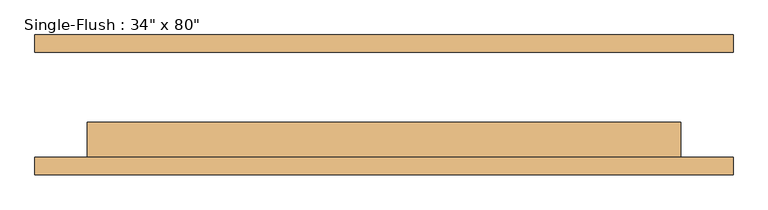
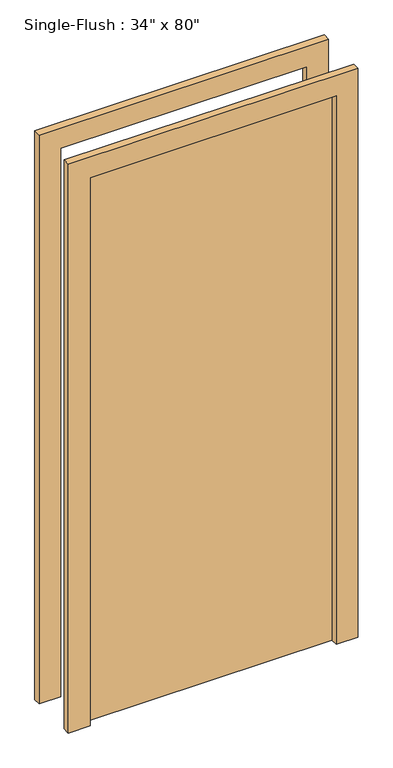
"""IFC4 building model written with IfcOpenShell, lengths in millimetres: door geometry."""

from ifc_helpers import new_model, si_unit, frame, origin, origin_with_axes, place, context, project, spatial, polyline, outline, extrude, source, transform, mapped, element, save


def door_706f0888(model_context):
    return source(origin(), model_context, "Body", "SweptSolid", [
        extrude(outline(polyline([(2108.2, -508.0), (0.0, -508.0), (0.0, -431.8), (2032.0, -431.8), (2032.0, 431.8), (0.0, 431.8), (0.0, 508.0), (2108.2, 508.0), (2108.2, -508.0)])), frame((0.0, -101.6, 0.0), z_axis=(0.0, 1.0, 0.0), x_axis=(0.0, 0.0, 1.0)), (0.0, 0.0, 1.0), 25.4),
        extrude(outline(polyline([(2108.2, 508.0), (2108.2, -508.0), (0.0, -508.0), (0.0, -431.8), (2032.0, -431.8), (2032.0, 431.8), (0.0, 431.8), (0.0, 508.0), (2108.2, 508.0)])), frame((0.0, 76.2, 0.0), z_axis=(0.0, 1.0, 0.0), x_axis=(0.0, 0.0, 1.0)), (0.0, 0.0, 1.0), 25.4),
        extrude(outline(polyline([(431.8, -25.4), (431.8, -76.2), (-431.8, -76.2), (-431.8, -25.4), (431.8, -25.4)])), origin_with_axes(), (0.0, 0.0, 1.0), 2032.0),
    ])


if __name__ == "__main__":
    model = new_model("IFC4")
    model_context = context("Model", 3, world=origin())
    ifc_project = project(units=[si_unit("LENGTHUNIT", "METRE", prefix="MILLI")], contexts=[model_context])
    site = spatial("IfcSite", under=ifc_project)
    building = spatial("IfcBuilding", under=site)
    placement = place(None, origin())
    door_shape = door_706f0888(model_context)
    element("IfcDoor", 1, ObjectType="Single-Flush : 34\" x 80\"", at=placement, inside=building, context=model_context, shape_type="MappedRepresentation", body=[
        mapped(door_shape, transform((0.0, 0.0, 0.0), x_axis=(1.0, 0.0, 0.0), y_axis=(0.0, 1.0, 0.0), z_axis=(0.0, 0.0, 1.0))),
    ])
    save(model, "model.ifc")

# Revit data of these elements
# Type "Single-Flush : 34\" x 80\""
#   Type Mark = "7"
#   Construction Type Id = "MDOOR"
#   Assembly Code = "C1020"
#   Analytic Construction = "Metal"
#   Thickness = 0' - 2"
#   Heat Transfer Coefficient (U) = 0.651978 BTU/(h·ft²·°F)
#   Height = 6' - 8"
#   Trim Projection Ext = 0' - 1"
#   Trim Projection Int = 0' - 1"
#   Trim Width = 0' - 3"
#   Width = 2' - 10"
#   Define Thermal Properties by = 1
#   Door Material = Door - Panel
#   Frame Material = Door - Frame
#   Visual Light Transmittance = 0
#   Solar Heat Gain Coefficient = 0
#   Function = (empty or 0)
#   Wall Closure = (empty or 0)
# Element 1 (IfcDoor, "Single-Flush : 34\" x 80\"")
#   Materials on its faces: "Door - Frame", "Door - Panel"
# Materials
#   "Door - Panel": class "Wood", colour RGB 210 159 95, transparency 0
#   "Door - Frame": colour RGB 118 70 51, transparency 0
